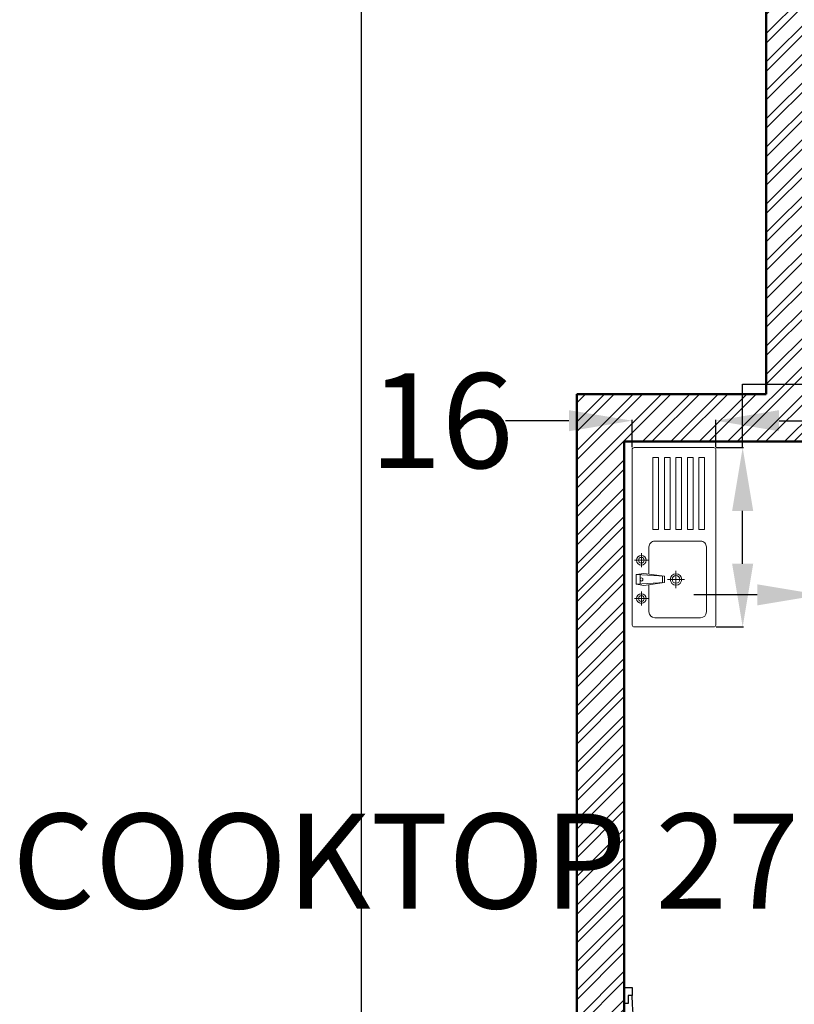
# Model space of a CAD drawing. Units: inches. Extents: x -90 to 536, y -553 to 299.
# Tile 11 of 27: x -68 to 79, y -339 to -153. Entities that reach past the tile are written whole.
import ezdxf

# ---------------------------------------------------------------- set-up
doc = ezdxf.new("R2010")
doc.units = ezdxf.units.IN
for name, color, linetype, lineweight in [('A-ANNO-DIMS', 2, 'Continuous', 18), ('A-DOOR', 4, 'Continuous', 25), ('A-FLOR-FIXT', 8, 'Continuous', 18), ('A-WALL-PATT', 252, 'Continuous', 13), ('Outer Wall', 1, 'Continuous', 50)]:
    doc.layers.add(name, color=color, linetype=linetype, lineweight=lineweight)
doc.styles.get("Standard").update_dxf_attribs({"font": 'arial.ttf'})
doc.dimstyles.get("Standard").update_dxf_attribs({"dimtxt": 18, "dimasz": 12, "dimexe": 0.18, "dimexo": 0.0625, "dimgap": 0.09, "dimtad": 0, "dimtih": 1, "dimtoh": 1, "dimdec": 0, "dimzin": 0, "dimdsep": 46, "dimlunit": 3, "dimtxsty": 'Standard', "dimcen": 0.09, "dimadec": 0, "dimazin": 0, "dimtfac": 1, "dimtdec": 0, "dimtofl": 0, "dimtmove": 0, "dimatfit": 3, "dimfxl": 1, "dimtolj": 1, "dimtzin": 0, "dimarcsym": 0})

# ---------------------------------------------------------------- blocks, each defined once
blk = doc.blocks.new('A$C7C492201')
for p, q in [((0, 10), (0, 426.6)), ((10, 436.6), (927.3, 436.6)), ((148.5, 425.2), (148.5, 352.2)), ((223.5, 415), (217, 376.2)), ((223.5, 415), (231.8, 268.5)), ((223.5, 415), (248.5, 415)), ((273.5, 415), (248.5, 415)), ((273.5, 415), (265.2, 268.5)), ((273.5, 415), (279.9, 376.2)), ((348.5, 425.2), (348.5, 352.2)), ((937.3, 10), (937.3, 426.6)), ((111.9, 388.7), (185, 388.7)), ((217, 376.2), (231.8, 268.5)), ((224.6, 395.4), (248.5, 395.4)), ((272.3, 395.4), (248.5, 395.4)), ((279.9, 376.2), (265.2, 268.5)), ((311.9, 388.7), (385, 388.7)), ((48.5, 318.8), (48.5, 78.8)), ((220.8, 348.8), (78.5, 348.8)), ((418.5, 348.8), (276.2, 348.8)), ((448.5, 318.8), (448.5, 78.8)), ((509.1, 328.4), (509.1, 298.4)), ((509.1, 328.4), (885, 328.4)), ((885, 328.4), (885, 298.4)), ((231.3, 278.6), (248.5, 278.6)), ((231.8, 268.5), (248.5, 268.5)), ((265.6, 278.6), (248.5, 278.6)), ((265.2, 268.5), (248.5, 268.5)), ((509.1, 298.4), (885, 298.4)), ((509.1, 268.4), (509.1, 238.4)), ((509.1, 268.4), (885, 268.4)), ((885, 268.4), (885, 238.4)), ((203.4, 207.7), (293.5, 207.7)), ((248.5, 252.8), (248.5, 162.6)), ((509.1, 238.4), (885, 238.4)), ((509.1, 208.4), (885, 208.4)), ((509.1, 208.4), (509.1, 178.4)), ((885, 208.4), (885, 178.4)), ((509.1, 178.4), (885, 178.4)), ((509.1, 148.4), (509.1, 118.4)), ((509.1, 148.4), (885, 148.4)), ((509.1, 118.4), (885, 118.4)), ((885, 148.4), (885, 118.4)), ((509.1, 88.4), (509.1, 58.4)), ((509.1, 88.4), (885, 88.4)), ((509.1, 58.4), (885, 58.4)), ((885, 88.4), (885, 58.4)), ((927.3, 0), (10, 0)), ((418.5, 48.8), (78.5, 48.8))]:
    blk.add_line(p, q)
for centre, radius in [((148.5, 388.7), 25), ((348.5, 388.7), 25), ((148.5, 388.7), 15), ((348.5, 388.7), 15), ((248.5, 207.7), 30), ((248.5, 207.7), 20)]:
    blk.add_circle(centre, radius)
for centre, radius, start, end in [((10, 426.6), 10, 90, 180), ((927.3, 426.6), 10, 0, 90), ((247.3, 388), 7.19, 80.5252, 279.4748), ((249.6, 388), 7.19, 260.5252, 99.4748), ((78.5, 318.8), 30, 90, 180), ((418.5, 318.8), 30, 0, 90), ((78.5, 78.8), 30, 180, 270), ((418.5, 78.8), 30, 270, 0), ((10, 10), 10, 180, 270), ((927.3, 10), 10, 270, 0)]:
    blk.add_arc(centre, radius, start, end)
blk = doc.blocks.new('DOOR-36-A')
for points in [[(35.25, 37.5), (35.25, 3), (34.5, 3), (34.5, 37.5)], [(0, 0), (1.5, 0), (1.5, 1.5), (0.75, 1.5), (0.75, 3), (0, 3)], [(36, 0), (34.5, 0), (34.5, 1.5), (35.25, 1.5), (35.25, 3), (36, 3)]]:
    blk.add_lwpolyline(points, close=True)
blk.add_arc((37.64, 1.5), 36.14, 94.9791, 180)
blk = doc.blocks.new('*D45')
at = {"layer": 'A-ANNO-DIMS', "color": 0, "lineweight": -2, "transparency": 16777216}
for p, q in [((96.92, -312.07), (84.92, -312.07)), ((96.92, -316.13), (96.92, -311.89)), ((112.4, -312.07), (108.92, -312.07)), ((124.4, -316.13), (124.4, -311.89))]:
    blk.add_line(p, q, dxfattribs=at)
at = {"layer": 'A-ANNO-DIMS', "color": 0, "transparency": 16777216}
for points in [[(108.92, -310.07), (108.92, -314.07), (96.92, -312.07)], [(112.4, -310.07), (112.4, -314.07), (124.4, -312.07)]]:
    blk.add_solid(points, dxfattribs=at)
at = {"layer": 'Defpoints', "color": 0, "transparency": 16777216}
for p in [(96.92, -312.07), (96.92, -316.19), (124.4, -316.19)]:
    blk.add_point(p, dxfattribs=at)
at = {"layer": 'A-ANNO-DIMS', "color": 0, "transparency": 16777216, "insert": (5.68, -312.07), "char_height": 18, "attachment_point": 5}
blk.add_mtext('\\A1;COOKTOP 27', dxfattribs=at)
blk = doc.blocks.new('*D46')
at = {"layer": 'A-ANNO-DIMS', "color": 0, "lineweight": -2, "transparency": 16777216}
for p, q in [((92.8, -304.19), (92.8, -292.19)), ((96.86, -316.19), (92.62, -316.19)), ((96.86, -332.23), (92.62, -332.23)), ((92.8, -344.23), (92.8, -356.23)), ((92.8, -356.23), (80.8, -356.23))]:
    blk.add_line(p, q, dxfattribs=at)
at = {"layer": 'A-ANNO-DIMS', "color": 0, "transparency": 16777216}
for points in [[(90.8, -304.19), (94.8, -304.19), (92.8, -316.19)], [(90.8, -344.23), (94.8, -344.23), (92.8, -332.23)]]:
    blk.add_solid(points, dxfattribs=at)
at = {"layer": 'Defpoints', "color": 0, "transparency": 16777216}
for p in [(96.92, -316.19), (92.8, -332.23), (96.92, -332.23)]:
    blk.add_point(p, dxfattribs=at)
at = {"layer": 'A-ANNO-DIMS', "color": 0, "transparency": 16777216, "insert": (68.67, -356.23), "char_height": 18, "attachment_point": 5}
blk.add_mtext('\\A1;16', dxfattribs=at)
blk = doc.blocks.new('*D47')
at = {"layer": 'A-ANNO-DIMS', "color": 0, "lineweight": -2, "transparency": 16777216}
for p, q in [((69.57, -233.68), (69.57, -221.68)), ((69.57, -221.68), (81.57, -221.68)), ((64.53, -233.68), (69.75, -233.68)), ((69.57, -255.69), (69.57, -245.68)), ((64.53, -267.69), (69.75, -267.69))]:
    blk.add_line(p, q, dxfattribs=at)
at = {"layer": 'A-ANNO-DIMS', "color": 0, "transparency": 16777216}
for points in [[(67.57, -245.68), (71.57, -245.68), (69.57, -233.68)], [(67.57, -255.69), (71.57, -255.69), (69.57, -267.69)]]:
    blk.add_solid(points, dxfattribs=at)
at = {"layer": 'Defpoints', "color": 0, "transparency": 16777216}
for p in [(64.47, -233.68), (69.57, -233.68), (64.47, -267.69)]:
    blk.add_point(p, dxfattribs=at)
at = {"layer": 'A-ANNO-DIMS', "color": 0, "transparency": 16777216, "insert": (127.31, -221.68), "char_height": 18, "attachment_point": 5}
blk.add_mtext('\\A1;SINK 34', dxfattribs=at)
blk = doc.blocks.new('*D48')
at = {"layer": 'A-ANNO-DIMS', "color": 0, "lineweight": -2, "transparency": 16777216}
for p, q in [((36.62, -228.58), (24.62, -228.58)), ((48.62, -233.62), (48.62, -228.4)), ((64.47, -233.62), (64.47, -228.4)), ((76.47, -228.58), (88.47, -228.58))]:
    blk.add_line(p, q, dxfattribs=at)
at = {"layer": 'A-ANNO-DIMS', "color": 0, "transparency": 16777216}
for points in [[(36.62, -226.58), (36.62, -230.58), (48.62, -228.58)], [(76.47, -226.58), (76.47, -230.58), (64.47, -228.58)]]:
    blk.add_solid(points, dxfattribs=at)
at = {"layer": 'Defpoints', "color": 0, "transparency": 16777216}
for p in [(48.62, -228.58), (48.62, -233.68), (64.47, -233.68)]:
    blk.add_point(p, dxfattribs=at)
at = {"layer": 'A-ANNO-DIMS', "color": 0, "transparency": 16777216, "insert": (12.5, -228.58), "char_height": 18, "attachment_point": 5}
blk.add_mtext('\\A1;16', dxfattribs=at)
blk = doc.blocks.new('*D50')
at = {"layer": 'A-ANNO-DIMS', "color": 0, "lineweight": -2, "transparency": 16777216}
for p, q in [((84.33, -257.38), (84.33, -261.78)), ((111, -257.38), (111, -261.78)), ((72.33, -261.6), (60.33, -261.6)), ((123, -261.6), (135, -261.6))]:
    blk.add_line(p, q, dxfattribs=at)
at = {"layer": 'A-ANNO-DIMS', "color": 0, "transparency": 16777216}
for points in [[(72.33, -259.6), (72.33, -263.6), (84.33, -261.6)], [(123, -259.6), (123, -263.6), (111, -261.6)]]:
    blk.add_solid(points, dxfattribs=at)
at = {"layer": 'Defpoints', "color": 0, "transparency": 16777216}
for p in [(84.33, -257.31), (111, -257.31), (111, -261.6)]:
    blk.add_point(p, dxfattribs=at)
at = {"layer": 'A-ANNO-DIMS', "color": 0, "transparency": 16777216, "insert": (97.67, -261.6), "char_height": 18, "attachment_point": 5}
blk.add_mtext('\\A1;27', dxfattribs=at)
blk = doc.blocks.new('*D54')
at = {"layer": 'A-ANNO-DIMS', "color": 0, "lineweight": -2, "transparency": 16777216}
for p, q in [((113.07, 249.45), (-2.85, 249.45)), ((-2.67, 237.45), (-2.67, -117.77)), ((-2.67, -491.55), (-2.67, -136.34)), ((38.07, -503.55), (-2.85, -503.55))]:
    blk.add_line(p, q, dxfattribs=at)
at = {"layer": 'A-ANNO-DIMS', "color": 0, "transparency": 16777216}
for points in [[(-4.67, 237.45), (-0.67, 237.45), (-2.67, 249.45)], [(-4.67, -491.55), (-0.67, -491.55), (-2.67, -503.55)]]:
    blk.add_solid(points, dxfattribs=at)
at = {"layer": 'Defpoints', "color": 0, "transparency": 16777216}
for p in [(-2.67, 249.45), (113.13, 249.45), (38.13, -503.55)]:
    blk.add_point(p, dxfattribs=at)
at = {"layer": 'A-ANNO-DIMS', "color": 0, "transparency": 16777216, "insert": (-2.67, -127.05), "char_height": 18, "attachment_point": 5}
blk.add_mtext('\\A1;753', dxfattribs=at)

msp = doc.modelspace()

# ---------------------------------------------------------------- hatches: boundary and pattern name
at = {"layer": 'A-WALL-PATT'}
h = msp.add_hatch(dxfattribs=at)
h.set_pattern_fill('ANSI32', color=256, scale=0.4)
h.set_pattern_definition([(45, (-88.8105, -603.6155), (-2.694077, 2.694077), []), (45, (-87.0145, -603.6155), (-2.694077, 2.694077), [])])
h.paths.add_polyline_path([(285.1317, 246.4462), (131.1317, 246.4462), (131.1317, 237.4462), (285.1317, 237.4462)])
h.paths.add_polyline_path([(122.1317, 237.4462), (113.1317, 237.4462), (113.1317, 152.4462), (122.1317, 152.4462), (122.1317, 166.4704)])
h.paths.add_polyline_path([(303.1317, 237.4462), (294.1317, 237.4462), (294.1317, 152.4462), (303.1317, 152.4462)])
h.paths.add_polyline_path([(47.1317, 91.9277), (38.1317, 91.9277), (38.1317, -6.5538), (77.1317, -6.5538), (77.1317, 2.4462), (70.5655, 2.4462), (47.1317, 2.4462)])
h.paths.add_polyline_path([(83.052, -61.5538), (47.1317, -61.5538), (47.1317, -24.5538), (38.1317, -24.5538), (38.1317, -70.5538), (74.052, -70.5538), (74.052, -223.5538), (38.1317, -223.5538), (38.1317, -503.5538), (92.1317, -503.5538), (92.1317, -437.5538), (191.1317, -437.5538), (191.1317, -428.5538), (83.1317, -428.5538), (83.1317, -494.5538), (47.1317, -494.5538), (47.1317, -232.5538), (83.052, -232.5538), (83.052, -70.5538)])
h.paths.add_polyline_path([(407.1317, -63.5538), (381.1317, -63.5538), (381.1317, 91.9277), (372.1317, 91.9277), (372.1317, 32.8805), (372.1317, -63.5538), (306.5745, -63.5538), (237.1317, -63.5538), (237.1317, -38.5538), (233.1317, -38.5538), (233.1317, -71.5538), (398.1317, -71.5538), (398.1317, -152.5538), (233.1317, -152.5538), (233.1317, -161.5538), (398.1317, -161.5538), (398.1317, -368.5538), (233.1317, -368.5538), (233.1317, -377.5538), (407.1317, -377.5538), (407.1317, -161.5538)])
h.paths.add_polyline_path([(261.1317, -422.5538), (252.1317, -422.5538), (252.1317, -428.5538), (233.1317, -428.5538), (233.1317, -437.5538), (261.1317, -437.5538)])
h.paths.add_polyline_path([(191.1317, -368.5538), (180.1317, -368.5538), (180.1317, -335.5538), (131.5919, -335.5538), (131.5919, -344.5538), (171.1317, -344.5538), (171.1317, -392.5538), (180.1317, -392.5538), (180.1317, -377.5538), (191.1317, -377.5538)], flags=17)
h.paths.add_polyline_path([(180.1317, -223.5538), (152.1317, -223.5538), (152.1317, -227.5538), (176.1317, -227.5538), (176.1317, -335.5538), (180.1317, -335.5538)], flags=17)
h.paths.add_polyline_path([(131.5919, -335.5538), (83.1317, -335.5538), (83.1317, -339.5538), (83.1317, -392.5538), (87.1317, -392.5538), (87.1317, -339.5538), (131.5919, -339.5538)], flags=17)
h.paths.add_polyline_path([(197.1317, 2.4462), (77.1317, 2.4462), (77.1317, -1.5538), (113.1317, -1.5538), (113.1317, -71.5538), (181.1317, -71.5538), (181.1317, -67.5538), (117.1317, -67.5538), (117.1317, -1.5538), (177.1317, -1.5538), (177.1317, -37.5538), (181.1317, -37.5538), (181.1317, -1.5538), (197.1317, -1.5538)])
h.paths.add_polyline_path([(173.1317, 138.4462), (122.1317, 138.4462), (122.1317, 134.4462), (173.1317, 134.4462)])
h.paths.add_polyline_path([(213.1317, 237.4462), (209.1317, 237.4462), (209.1317, 134.4462), (233.1317, 134.4462), (233.1317, 68.8889), (233.1317, -2.5538), (237.1317, -2.5538), (237.1317, 134.4462), (258.1317, 134.4462), (258.1317, 138.4462), (213.1317, 138.4462)])

# ---------------------------------------------------------------- linework, layer by layer
at = {"layer": 'Outer Wall'}
for p, q in [((74.052, -70.5538), (74.052, -223.5538)), ((74.052, -223.5538), (38.1317, -223.5538)), ((38.1317, -223.5538), (38.1317, -503.5538)), ((47.1317, -232.5538), (47.1317, -494.5538)), ((83.052, -232.5538), (47.1317, -232.5538))]:
    msp.add_line(p, q, dxfattribs=at)

# ---------------------------------------------------------------- block references
at = {"layer": 'A-DOOR', "extrusion": (0, 0, -1), "zscale": -1, "rotation": 180}
msp.add_blockref('DOOR-36-A', (-47.1317, -336.0538), dxfattribs=at)
at = {"layer": 'A-FLOR-FIXT', "xscale": 0.0362851414289068, "yscale": 0.0362851414289068, "zscale": 0.0362851414289068, "rotation": 89.99999999999999}
msp.add_blockref('A$C7C492201', (64.4668, -267.6933), dxfattribs=at)

# ---------------------------------------------------------------- dimensions: what is measured, and where the dimension line sits
at = {"layer": 'A-ANNO-DIMS'}
for base, p1, p2, angle, picture, middle in [((-2.6677, 249.4462), (38.1317, -503.5538), (113.1317, 249.4462), 90, '*D54', (-2.6677, -127.0538)), ((48.6244, -228.5837), (64.4668, -233.6849), (48.6244, -233.6849), 180, '*D48', (12.4955, -228.5837)), ((92.7963, -332.2258), (96.9187, -316.194), (96.9187, -332.2258), 270, '*D46', (68.6674, -356.2258))]:
    dim = msp.add_linear_dim(base=base, p1=p1, p2=p2, angle=angle, dimstyle='Standard', override={"dimdec": 0, "dimlfac": 1, "dimrnd": 0, "dimzin": 0, "dimdsep": 46, "dimlunit": 2}, dxfattribs=at)
    dim.commit()
    dim.dimension.update_dxf_attribs({"geometry": picture, "text_midpoint": middle})
for base, p1, p2, angle, text, picture, middle in [((69.5681, -233.6849), (64.4668, -267.6933), (64.4668, -233.6849), 90, 'SINK <>', '*D47', (127.3088, -221.6849)), ((96.9187, -312.0716), (124.4017, -316.194), (96.9187, -316.194), 180, 'COOKTOP <>', '*D45', (5.6766, -312.0716))]:
    dim = msp.add_linear_dim(base=base, p1=p1, p2=p2, angle=angle, text=text, dimstyle='Standard', override={"dimdec": 0, "dimlfac": 1, "dimrnd": 0, "dimzin": 0, "dimdsep": 46, "dimlunit": 2}, dxfattribs=at)
    dim.commit()
    dim.dimension.update_dxf_attribs({"geometry": picture, "text_midpoint": middle})
dim = msp.add_linear_dim(base=(110.9988, -261.6002), p1=(84.3335, -257.3147), p2=(110.9988, -257.3147), dimstyle='Standard', override={"dimdec": 0, "dimlfac": 1, "dimrnd": 0, "dimzin": 0, "dimdsep": 46, "dimlunit": 2}, dxfattribs=at)
dim.commit()
dim.dimension.update_dxf_attribs({"geometry": '*D50', "text_midpoint": (97.6662, -261.6002)})

doc.saveas('drawing.dxf')
